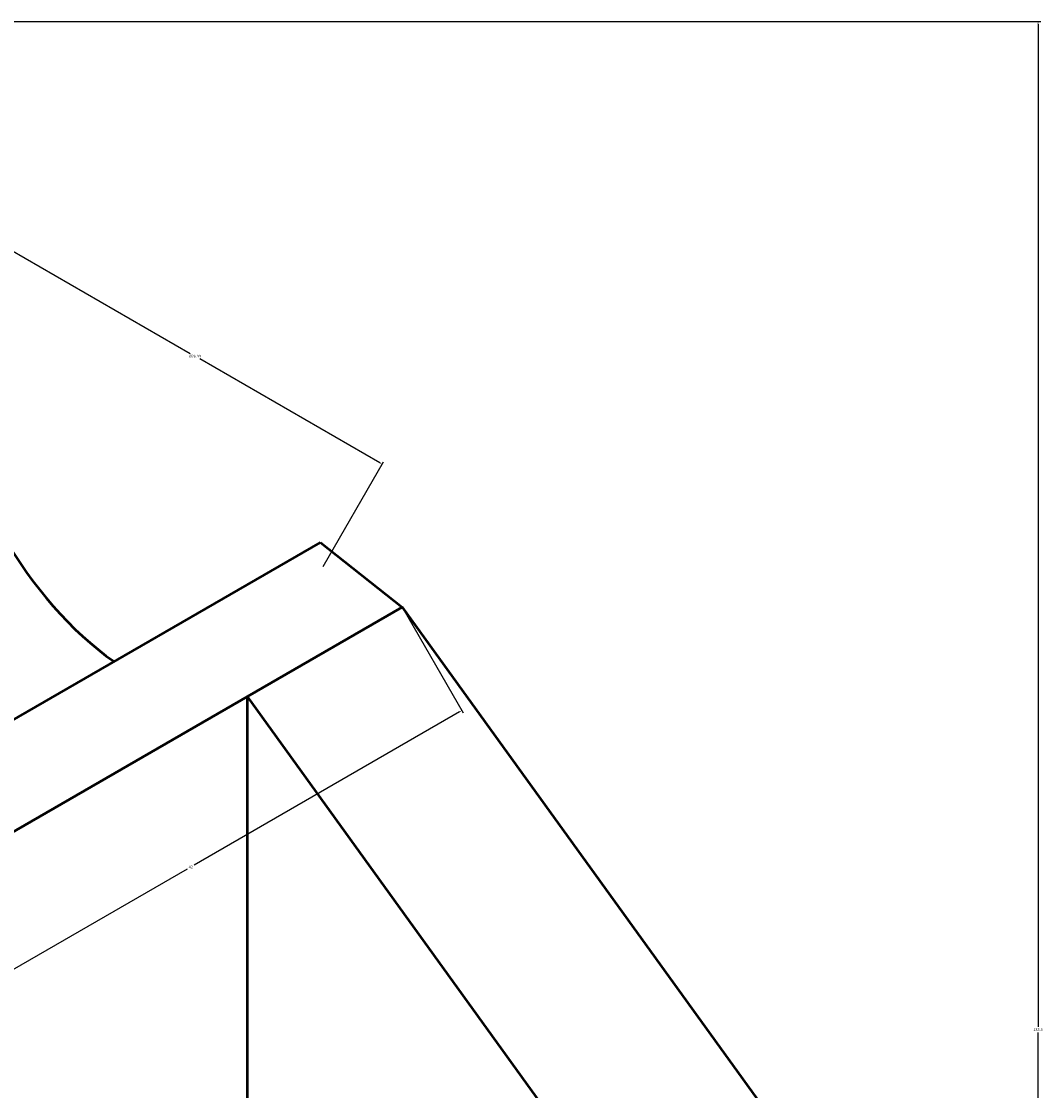
# Model space of a CAD drawing. Units: millimetres. Extents: x 2919 to 3075, y 2801 to 2951.
# Tile 14 of 14: x 3006 to 3075, y 2872 to 2944. Entities that reach past the tile are written whole.
import ezdxf

# ---------------------------------------------------------------- set-up
doc = ezdxf.new("R2010")
doc.units = ezdxf.units.MM
doc.layers.add('M-DIMS', color=2, linetype='Continuous', lineweight=18)
doc.layers.add('M-OUTL', color=7, linetype='Continuous', lineweight=50)
doc.styles.get("Standard").update_dxf_attribs({"font": 'arial.ttf'})
doc.dimstyles.get("Standard").update_dxf_attribs({"dimtxt": 0.18, "dimasz": 0.18, "dimexe": 0.18, "dimexo": 0.0625, "dimgap": 0.09, "dimtad": 0, "dimtih": 1, "dimtoh": 1, "dimdec": 4, "dimzin": 0, "dimdsep": 46, "dimtxsty": 'Standard', "dimcen": 0.09, "dimadec": 0, "dimazin": 0, "dimtfac": 1, "dimtdec": 4, "dimtofl": 0, "dimtmove": 0, "dimatfit": 3, "dimfxl": 1, "dimtolj": 1, "dimtzin": 0, "dimarcsym": 0})

# ---------------------------------------------------------------- blocks, each defined once
blk = doc.blocks.new('*D1')
at = {"layer": 'Defpoints', "color": 0, "transparency": 16777216}
for p in [(2987.323, 2944.203), (3074.337, 2944.203), (3010.912, 2808.893)]:
    blk.add_point(p, dxfattribs=at)
at = {"layer": 'M-DIMS', "color": 0, "lineweight": -2, "transparency": 16777216}
for p, q in [((2987.386, 2944.203), (3074.517, 2944.203)), ((3074.337, 2944.023), (3074.337, 2876.73)), ((3074.337, 2809.073), (3074.337, 2876.366)), ((3010.974, 2808.893), (3074.517, 2808.893))]:
    blk.add_line(p, q, dxfattribs=at)
at = {"layer": 'M-DIMS', "color": 0, "transparency": 16777216}
for points in [[(3074.307, 2944.023), (3074.367, 2944.023), (3074.337, 2944.203)], [(3074.307, 2809.073), (3074.367, 2809.073), (3074.337, 2808.893)]]:
    blk.add_solid(points, dxfattribs=at)
at = {"layer": 'M-DIMS', "color": 0, "transparency": 16777216, "insert": (3074.337, 2876.548), "char_height": 0.18, "attachment_point": 5}
blk.add_mtext('\\A1;135.3', dxfattribs=at)
blk = doc.blocks.new('*D12')
at = {"layer": 'Defpoints', "color": 0, "transparency": 16777216}
for p in [(3031.696, 2904.893), (2995.323, 2883.893), (2999.323, 2876.965)]:
    blk.add_point(p, dxfattribs=at)
at = {"layer": 'M-DIMS', "color": 0, "lineweight": -2, "transparency": 16777216}
for p, q in [((3031.727, 2904.839), (3035.786, 2897.809)), ((3035.54, 2897.875), (3017.731, 2887.593)), ((2999.479, 2877.055), (3017.288, 2887.337)), ((2995.354, 2883.839), (2999.413, 2876.809))]:
    blk.add_line(p, q, dxfattribs=at)
at = {"layer": 'M-DIMS', "color": 0, "transparency": 16777216}
for points in [[(3035.525, 2897.901), (3035.555, 2897.849), (3035.696, 2897.965)], [(2999.464, 2877.081), (2999.494, 2877.029), (2999.323, 2876.965)]]:
    blk.add_solid(points, dxfattribs=at)
at = {"layer": 'M-DIMS', "color": 0, "transparency": 16777216, "insert": (3017.51, 2887.465), "char_height": 0.18, "attachment_point": 5}
blk.add_mtext('\\A1;42', dxfattribs=at)
blk = doc.blocks.new('*D18')
at = {"layer": 'Defpoints', "color": 0, "transparency": 16777216}
for p in [(3001.241, 2922.061), (3030.348, 2914.493), (3026.348, 2907.565)]:
    blk.add_point(p, dxfattribs=at)
at = {"layer": 'M-DIMS', "color": 0, "lineweight": -2, "transparency": 16777216}
for p, q in [((3001.272, 2922.115), (3005.331, 2929.145)), ((3005.397, 2928.899), (3017.471, 2921.928)), ((3030.192, 2914.583), (3018.118, 2921.554)), ((3026.379, 2907.619), (3030.438, 2914.649))]:
    blk.add_line(p, q, dxfattribs=at)
at = {"layer": 'M-DIMS', "color": 0, "transparency": 16777216}
for points in [[(3005.412, 2928.925), (3005.382, 2928.873), (3005.241, 2928.989)], [(3030.207, 2914.609), (3030.177, 2914.557), (3030.348, 2914.493)]]:
    blk.add_solid(points, dxfattribs=at)
at = {"layer": 'M-DIMS', "color": 0, "transparency": 16777216, "insert": (3017.794, 2921.741), "char_height": 0.18, "attachment_point": 5}
blk.add_mtext('\\A1;%%c28.99', dxfattribs=at)

msp = doc.modelspace()

# ---------------------------------------------------------------- linework, layer by layer
at = {"layer": 'M-OUTL'}
for p, q in [((2989.8305, 2888.2326), (3026.2035, 2909.2326)), ((3026.2035, 2909.2326), (3031.6962, 2904.8932)), ((3021.3039, 2898.8932), (3031.6962, 2904.8932)), ((3031.6962, 2904.8932), (3066.3372, 2856.8932)), ((2995.3232, 2883.8932), (3021.3039, 2898.8932)), ((3021.3039, 2870.8932), (3021.3039, 2898.8932)), ((3055.9449, 2850.8932), (3021.3039, 2898.8932))]:
    msp.add_line(p, q, dxfattribs=at)
for start_param, end_param in [(4.0414742, 5.3833038), (6.1286242, 6.1409334)]:
    msp.add_ellipse((3013.7944, 2914.8129), major_axis=(8.8766, -15.3748), ratio=0.5773503, start_param=start_param, end_param=end_param, dxfattribs=at)

# ---------------------------------------------------------------- dimensions: what is measured, and where the dimension line sits
at = {"layer": 'M-DIMS'}
for base, p1, p2, angle, override, picture, middle in [((3074.3372, 2944.2026), (3010.9116, 2808.8932), (2987.3232, 2944.2026), 90, {"dimdec": 1, "dimlfac": 1, "dimrnd": 0, "dimzin": 0, "dimdsep": 46, "dimlunit": 2}, '*D1', (3074.3372, 2876.5479)), ((2999.3232, 2876.965), (3031.6962, 2904.8932), (2995.3232, 2883.8932), 210, {"dimdec": 0, "dimlfac": 1, "dimrnd": 0, "dimzin": 0, "dimdsep": 46, "dimlunit": 2}, '*D12', (3017.5097, 2887.465))]:
    dim = msp.add_linear_dim(base=base, p1=p1, p2=p2, angle=angle, dimstyle='Standard', override=override, dxfattribs=at)
    dim.commit()
    dim.dimension.update_dxf_attribs({"geometry": picture, "text_midpoint": middle})
dim = msp.add_linear_dim(base=(3030.3479, 2914.4934), p1=(3001.241, 2922.0607), p2=(3026.3479, 2907.5652), angle=330, text='%%c<>', dimstyle='Standard', override={"dimdec": 2, "dimlfac": 1, "dimrnd": 0, "dimzin": 0, "dimdsep": 46, "dimlunit": 2}, dxfattribs=at)
dim.commit()
dim.dimension.update_dxf_attribs({"geometry": '*D18', "text_midpoint": (3017.7944, 2921.7411)})

doc.saveas('drawing.dxf')
